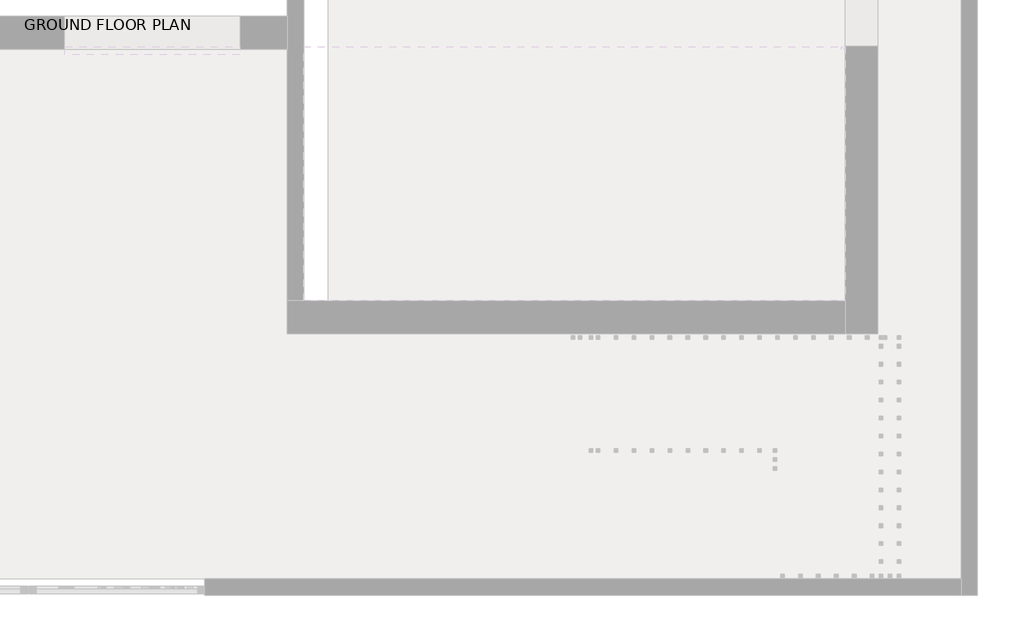
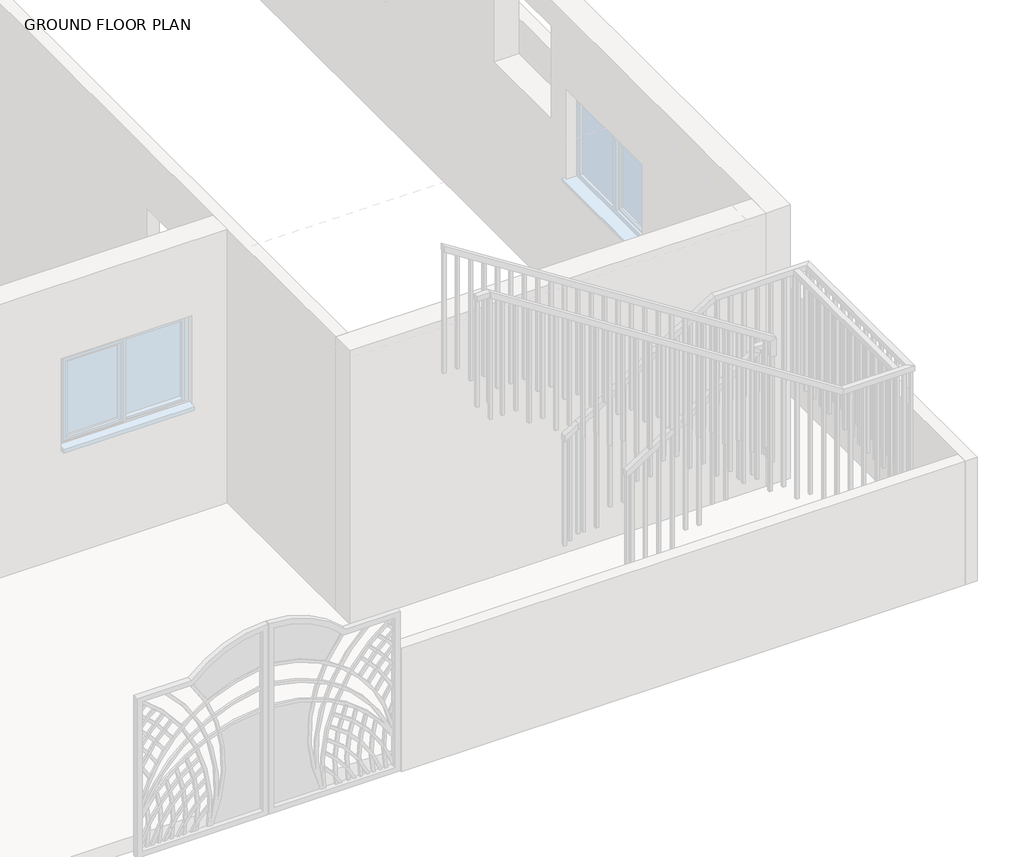
# One storey, part 8 of 23: 2 railings.
"""IFC4 building model written with IfcOpenShell, lengths in millimetres."""

from ifc_helpers import new_model, si_unit, frame, origin, place, context, project, spatial, polyline, outline, extrude, faceted_brep, element, save

model = new_model("IFC4")

# Units and contexts
model_context = context("Model", 3, world=origin())
ifc_project = project(units=[si_unit("LENGTHUNIT", "METRE", prefix="MILLI")], contexts=[model_context])

# Site, building, storey
site = spatial("IfcSite", under=ifc_project)
building = spatial("IfcBuilding", under=site)
storey = spatial("IfcBuildingStorey", under=building, Name="GROUND FLOOR PLAN", Elevation=487.68)

# Railings
placement = place(None, origin())
element("IfcRailing", 1, ObjectType="1100mm", at=placement, inside=storey, context=model_context, shape_type="SolidModel", body=[
    faceted_brep([(-8680.149573, -10220.0521308, 1912.8), (-8680.149573, -10220.0521308, 1853.4423995), (-8680.149573, -10270.0521308, 1853.4423995), (-8680.149573, -10270.0521308, 1912.8), (-7409.7306254, -10220.0521308, 2725.6), (-7395.1045513, -10220.0521308, 2675.6), (-7395.1045513, -10270.0521308, 2675.6), (-7409.7306254, -10270.0521308, 2725.6), (-6495.8132565, -10220.0521308, 2725.6), (-6495.8132565, -10220.0521308, 2675.6), (-6545.8132565, -10270.0521308, 2675.6), (-6545.8132565, -10270.0521308, 2725.6), (-6495.8132565, -11933.6860066, 2725.6), (-6495.8132565, -11933.6860066, 2675.6), (-6545.8132565, -11883.6860066, 2675.6), (-6545.8132565, -11883.6860066, 2725.6), (-7155.718398, -11933.6860066, 2725.6), (-7170.3479429, -11933.6860066, 2675.6), (-7170.3479429, -11883.6860066, 2675.6), (-7155.718398, -11883.6860066, 2725.6), (-10457.8773536, -11933.6860066, 4838.88), (-10457.8773536, -11883.6860066, 4838.88), (-10457.8773536, -11883.6860066, 4779.517542), (-10457.8773536, -11933.6860066, 4779.517542)], [[[0, 1, 2, 3]], [[1, 0, 4, 5]], [[2, 1, 5, 6]], [[3, 2, 6, 7]], [[0, 3, 7, 4]], [[5, 4, 8, 9]], [[6, 5, 9, 10]], [[7, 6, 10, 11]], [[4, 7, 11, 8]], [[9, 8, 12, 13]], [[10, 9, 13, 14]], [[11, 10, 14, 15]], [[8, 11, 15, 12]], [[13, 12, 16, 17]], [[14, 13, 17, 18]], [[15, 14, 18, 19]], [[12, 15, 19, 16]], [[20, 21, 22, 23]], [[17, 16, 20, 23]], [[18, 17, 23, 22]], [[19, 18, 22, 21]], [[16, 19, 21, 20]]]),
    extrude(outline(polyline([(4691.8007425, -10320.8132565), (4707.7999723, -10345.8132565), (3576.32, -10345.8132565), (3576.32, -10320.8132565), (4691.8007425, -10320.8132565)])), frame((0.0, -11921.1860066, 0.0), z_axis=(0.0, 1.0, 0.0), x_axis=(0.0, 0.0, 1.0)), (0.0, 0.0, 1.0), 25.0),
    extrude(outline(polyline([(4611.8045935, -10195.8132565), (4627.8038233, -10220.8132565), (3576.32, -10220.8132565), (3576.32, -10195.8132565), (4611.8045935, -10195.8132565)])), frame((0.0, -11921.1860066, 0.0), z_axis=(0.0, 1.0, 0.0), x_axis=(0.0, 0.0, 1.0)), (0.0, 0.0, 1.0), 25.0),
    extrude(outline(polyline([(4531.8084444, -10070.8132565), (4547.8076742, -10095.8132565), (3413.76, -10095.8132565), (3413.76, -10070.8132565), (4531.8084444, -10070.8132565)])), frame((0.0, -11921.1860066, 0.0), z_axis=(0.0, 1.0, 0.0), x_axis=(0.0, 0.0, 1.0)), (0.0, 0.0, 1.0), 25.0),
    extrude(outline(polyline([(4451.8122954, -9945.8132565), (4467.8115252, -9970.8132565), (3413.76, -9970.8132565), (3413.76, -9945.8132565), (4451.8122954, -9945.8132565)])), frame((0.0, -11921.1860066, 0.0), z_axis=(0.0, 1.0, 0.0), x_axis=(0.0, 0.0, 1.0)), (0.0, 0.0, 1.0), 25.0),
    extrude(outline(polyline([(4371.8161463, -9820.8132565), (4387.8153761, -9845.8132565), (3251.2, -9845.8132565), (3251.2, -9820.8132565), (4371.8161463, -9820.8132565)])), frame((0.0, -11921.1860066, 0.0), z_axis=(0.0, 1.0, 0.0), x_axis=(0.0, 0.0, 1.0)), (0.0, 0.0, 1.0), 25.0),
    extrude(outline(polyline([(4291.8423995, -9695.8132565), (4307.8371231, -9720.8132565), (3251.2, -9720.8132565), (3251.2, -9695.8132565), (4291.8423995, -9695.8132565)])), frame((0.0, -11921.1860066, 0.0), z_axis=(0.0, 1.0, 0.0), x_axis=(0.0, 0.0, 1.0)), (0.0, 0.0, 1.0), 25.0),
    extrude(outline(polyline([(4211.8238482, -9570.8132565), (4227.823078, -9595.8132565), (3088.64, -9595.8132565), (3088.64, -9570.8132565), (4211.8238482, -9570.8132565)])), frame((0.0, -11921.1860066, 0.0), z_axis=(0.0, 1.0, 0.0), x_axis=(0.0, 0.0, 1.0)), (0.0, 0.0, 1.0), 25.0),
    extrude(outline(polyline([(4131.8276992, -9445.8132565), (4147.826929, -9470.8132565), (3088.64, -9470.8132565), (3088.64, -9445.8132565), (4131.8276992, -9445.8132565)])), frame((0.0, -11921.1860066, 0.0), z_axis=(0.0, 1.0, 0.0), x_axis=(0.0, 0.0, 1.0)), (0.0, 0.0, 1.0), 25.0),
    extrude(outline(polyline([(4051.8315501, -9320.8132565), (4067.8307799, -9345.8132565), (2926.08, -9345.8132565), (2926.08, -9320.8132565), (4051.8315501, -9320.8132565)])), frame((0.0, -11921.1860066, 0.0), z_axis=(0.0, 1.0, 0.0), x_axis=(0.0, 0.0, 1.0)), (0.0, 0.0, 1.0), 25.0),
    extrude(outline(polyline([(3971.835401, -9195.8132565), (3987.8346309, -9220.8132565), (2926.08, -9220.8132565), (2926.08, -9195.8132565), (3971.835401, -9195.8132565)])), frame((0.0, -11921.1860066, 0.0), z_axis=(0.0, 1.0, 0.0), x_axis=(0.0, 0.0, 1.0)), (0.0, 0.0, 1.0), 25.0),
    extrude(outline(polyline([(3891.839252, -9070.8132565), (3907.8384818, -9095.8132565), (2763.52, -9095.8132565), (2763.52, -9070.8132565), (3891.839252, -9070.8132565)])), frame((0.0, -11921.1860066, 0.0), z_axis=(0.0, 1.0, 0.0), x_axis=(0.0, 0.0, 1.0)), (0.0, 0.0, 1.0), 25.0),
    extrude(outline(polyline([(3811.8431029, -8945.8132565), (3827.8423328, -8970.8132565), (2763.52, -8970.8132565), (2763.52, -8945.8132565), (3811.8431029, -8945.8132565)])), frame((0.0, -11921.1860066, 0.0), z_axis=(0.0, 1.0, 0.0), x_axis=(0.0, 0.0, 1.0)), (0.0, 0.0, 1.0), 25.0),
    extrude(outline(polyline([(3731.8469539, -8820.8132565), (3747.8461837, -8845.8132565), (2600.96, -8845.8132565), (2600.96, -8820.8132565), (3731.8469539, -8820.8132565)])), frame((0.0, -11921.1860066, 0.0), z_axis=(0.0, 1.0, 0.0), x_axis=(0.0, 0.0, 1.0)), (0.0, 0.0, 1.0), 25.0),
    extrude(outline(polyline([(3651.8508048, -8695.8132565), (3667.8500347, -8720.8132565), (2600.96, -8720.8132565), (2600.96, -8695.8132565), (3651.8508048, -8695.8132565)])), frame((0.0, -11921.1860066, 0.0), z_axis=(0.0, 1.0, 0.0), x_axis=(0.0, 0.0, 1.0)), (0.0, 0.0, 1.0), 25.0),
    extrude(outline(polyline([(3571.8546558, -8570.8132565), (3587.8538856, -8595.8132565), (2438.4, -8595.8132565), (2438.4, -8570.8132565), (3571.8546558, -8570.8132565)])), frame((0.0, -11921.1860066, 0.0), z_axis=(0.0, 1.0, 0.0), x_axis=(0.0, 0.0, 1.0)), (0.0, 0.0, 1.0), 25.0),
    extrude(outline(polyline([(3491.8585067, -8445.8132565), (3507.8577365, -8470.8132565), (2438.4, -8470.8132565), (2438.4, -8445.8132565), (3491.8585067, -8445.8132565)])), frame((0.0, -11921.1860066, 0.0), z_axis=(0.0, 1.0, 0.0), x_axis=(0.0, 0.0, 1.0)), (0.0, 0.0, 1.0), 25.0),
    extrude(outline(polyline([(3411.8623577, -8320.8132565), (3427.8615875, -8345.8132565), (2275.84, -8345.8132565), (2275.84, -8320.8132565), (3411.8623577, -8320.8132565)])), frame((0.0, -11921.1860066, 0.0), z_axis=(0.0, 1.0, 0.0), x_axis=(0.0, 0.0, 1.0)), (0.0, 0.0, 1.0), 25.0),
    extrude(outline(polyline([(3331.8662086, -8195.8132565), (3347.8654384, -8220.8132565), (2275.84, -8220.8132565), (2275.84, -8195.8132565), (3331.8662086, -8195.8132565)])), frame((0.0, -11921.1860066, 0.0), z_axis=(0.0, 1.0, 0.0), x_axis=(0.0, 0.0, 1.0)), (0.0, 0.0, 1.0), 25.0),
    extrude(outline(polyline([(3251.8700596, -8070.8132565), (3267.8692894, -8095.8132565), (2113.28, -8095.8132565), (2113.28, -8070.8132565), (3251.8700596, -8070.8132565)])), frame((0.0, -11921.1860066, 0.0), z_axis=(0.0, 1.0, 0.0), x_axis=(0.0, 0.0, 1.0)), (0.0, 0.0, 1.0), 25.0),
    extrude(outline(polyline([(3171.8739105, -7945.8132565), (3187.8731403, -7970.8132565), (2113.28, -7970.8132565), (2113.28, -7945.8132565), (3171.8739105, -7945.8132565)])), frame((0.0, -11921.1860066, 0.0), z_axis=(0.0, 1.0, 0.0), x_axis=(0.0, 0.0, 1.0)), (0.0, 0.0, 1.0), 25.0),
    extrude(outline(polyline([(3091.8777615, -7820.8132565), (3107.8769913, -7845.8132565), (1950.72, -7845.8132565), (1950.72, -7820.8132565), (3091.8777615, -7820.8132565)])), frame((0.0, -11921.1860066, 0.0), z_axis=(0.0, 1.0, 0.0), x_axis=(0.0, 0.0, 1.0)), (0.0, 0.0, 1.0), 25.0),
    extrude(outline(polyline([(3011.8816124, -7695.8132565), (3027.8808422, -7720.8132565), (1950.72, -7720.8132565), (1950.72, -7695.8132565), (3011.8816124, -7695.8132565)])), frame((0.0, -11921.1860066, 0.0), z_axis=(0.0, 1.0, 0.0), x_axis=(0.0, 0.0, 1.0)), (0.0, 0.0, 1.0), 25.0),
    extrude(outline(polyline([(2931.8854634, -7570.8132565), (2947.8846932, -7595.8132565), (1788.16, -7595.8132565), (1788.16, -7570.8132565), (2931.8854634, -7570.8132565)])), frame((0.0, -11921.1860066, 0.0), z_axis=(0.0, 1.0, 0.0), x_axis=(0.0, 0.0, 1.0)), (0.0, 0.0, 1.0), 25.0),
    extrude(outline(polyline([(2851.8893143, -7445.8132565), (2867.8885441, -7470.8132565), (1788.16, -7470.8132565), (1788.16, -7445.8132565), (2851.8893143, -7445.8132565)])), frame((0.0, -11921.1860066, 0.0), z_axis=(0.0, 1.0, 0.0), x_axis=(0.0, 0.0, 1.0)), (0.0, 0.0, 1.0), 25.0),
    extrude(outline(polyline([(2771.8931653, -7320.8132565), (2787.8923951, -7345.8132565), (1625.6, -7345.8132565), (1625.6, -7320.8132565), (2771.8931653, -7320.8132565)])), frame((0.0, -11921.1860066, 0.0), z_axis=(0.0, 1.0, 0.0), x_axis=(0.0, 0.0, 1.0)), (0.0, 0.0, 1.0), 25.0),
    extrude(outline(polyline([(2691.8970162, -7195.8132565), (2707.896246, -7220.8132565), (1625.6, -7220.8132565), (1625.6, -7195.8132565), (2691.8970162, -7195.8132565)])), frame((0.0, -11921.1860066, 0.0), z_axis=(0.0, 1.0, 0.0), x_axis=(0.0, 0.0, 1.0)), (0.0, 0.0, 1.0), 25.0),
    extrude(outline(polyline([(-7070.8132565, -11921.1860066), (-7095.8132565, -11921.1860066), (-7095.8132565, -11896.1860066), (-7070.8132565, -11896.1860066), (-7070.8132565, -11921.1860066)])), frame((0.0, 0.0, 1625.6), z_axis=(0.0, 0.0, 1.0), x_axis=(1.0, 0.0, 0.0)), (0.0, 0.0, 1.0), 1050.0),
    extrude(outline(polyline([(-6945.8132565, -11921.1860066), (-6970.8132565, -11921.1860066), (-6970.8132565, -11896.1860066), (-6945.8132565, -11896.1860066), (-6945.8132565, -11921.1860066)])), frame((0.0, 0.0, 1625.6), z_axis=(0.0, 0.0, 1.0), x_axis=(1.0, 0.0, 0.0)), (0.0, 0.0, 1.0), 1050.0),
    extrude(outline(polyline([(-6820.8132565, -11921.1860066), (-6845.8132565, -11921.1860066), (-6845.8132565, -11896.1860066), (-6820.8132565, -11896.1860066), (-6820.8132565, -11921.1860066)])), frame((0.0, 0.0, 1625.6), z_axis=(0.0, 0.0, 1.0), x_axis=(1.0, 0.0, 0.0)), (0.0, 0.0, 1.0), 1050.0),
    extrude(outline(polyline([(-6695.8132565, -11921.1860066), (-6720.8132565, -11921.1860066), (-6720.8132565, -11896.1860066), (-6695.8132565, -11896.1860066), (-6695.8132565, -11921.1860066)])), frame((0.0, 0.0, 1625.6), z_axis=(0.0, 0.0, 1.0), x_axis=(1.0, 0.0, 0.0)), (0.0, 0.0, 1.0), 1050.0),
    extrude(outline(polyline([(-6570.8132565, -11921.1860066), (-6595.8132565, -11921.1860066), (-6595.8132565, -11896.1860066), (-6570.8132565, -11896.1860066), (-6570.8132565, -11921.1860066)])), frame((0.0, 0.0, 1625.6), z_axis=(0.0, 0.0, 1.0), x_axis=(1.0, 0.0, 0.0)), (0.0, 0.0, 1.0), 1050.0),
    extrude(outline(polyline([(-6508.3132565, -11795.0521308), (-6508.3132565, -11820.0521308), (-6533.3132565, -11820.0521308), (-6533.3132565, -11795.0521308), (-6508.3132565, -11795.0521308)])), frame((0.0, 0.0, 1625.6), z_axis=(0.0, 0.0, 1.0), x_axis=(1.0, 0.0, 0.0)), (0.0, 0.0, 1.0), 1050.0),
    extrude(outline(polyline([(-6508.3132565, -11670.0521308), (-6508.3132565, -11695.0521308), (-6533.3132565, -11695.0521308), (-6533.3132565, -11670.0521308), (-6508.3132565, -11670.0521308)])), frame((0.0, 0.0, 1625.6), z_axis=(0.0, 0.0, 1.0), x_axis=(1.0, 0.0, 0.0)), (0.0, 0.0, 1.0), 1050.0),
    extrude(outline(polyline([(-6508.3132565, -11545.0521308), (-6508.3132565, -11570.0521308), (-6533.3132565, -11570.0521308), (-6533.3132565, -11545.0521308), (-6508.3132565, -11545.0521308)])), frame((0.0, 0.0, 1625.6), z_axis=(0.0, 0.0, 1.0), x_axis=(1.0, 0.0, 0.0)), (0.0, 0.0, 1.0), 1050.0),
    extrude(outline(polyline([(-6508.3132565, -11420.0521308), (-6508.3132565, -11445.0521308), (-6533.3132565, -11445.0521308), (-6533.3132565, -11420.0521308), (-6508.3132565, -11420.0521308)])), frame((0.0, 0.0, 1625.6), z_axis=(0.0, 0.0, 1.0), x_axis=(1.0, 0.0, 0.0)), (0.0, 0.0, 1.0), 1050.0),
    extrude(outline(polyline([(-6508.3132565, -11295.0521308), (-6508.3132565, -11320.0521308), (-6533.3132565, -11320.0521308), (-6533.3132565, -11295.0521308), (-6508.3132565, -11295.0521308)])), frame((0.0, 0.0, 1625.6), z_axis=(0.0, 0.0, 1.0), x_axis=(1.0, 0.0, 0.0)), (0.0, 0.0, 1.0), 1050.0),
    extrude(outline(polyline([(-6508.3132565, -11170.0521308), (-6508.3132565, -11195.0521308), (-6533.3132565, -11195.0521308), (-6533.3132565, -11170.0521308), (-6508.3132565, -11170.0521308)])), frame((0.0, 0.0, 1625.6), z_axis=(0.0, 0.0, 1.0), x_axis=(1.0, 0.0, 0.0)), (0.0, 0.0, 1.0), 1050.0),
    extrude(outline(polyline([(-6508.3132565, -11045.0521308), (-6508.3132565, -11070.0521308), (-6533.3132565, -11070.0521308), (-6533.3132565, -11045.0521308), (-6508.3132565, -11045.0521308)])), frame((0.0, 0.0, 1625.6), z_axis=(0.0, 0.0, 1.0), x_axis=(1.0, 0.0, 0.0)), (0.0, 0.0, 1.0), 1050.0),
    extrude(outline(polyline([(-6508.3132565, -10920.0521308), (-6508.3132565, -10945.0521308), (-6533.3132565, -10945.0521308), (-6533.3132565, -10920.0521308), (-6508.3132565, -10920.0521308)])), frame((0.0, 0.0, 1625.6), z_axis=(0.0, 0.0, 1.0), x_axis=(1.0, 0.0, 0.0)), (0.0, 0.0, 1.0), 1050.0),
    extrude(outline(polyline([(-6508.3132565, -10795.0521308), (-6508.3132565, -10820.0521308), (-6533.3132565, -10820.0521308), (-6533.3132565, -10795.0521308), (-6508.3132565, -10795.0521308)])), frame((0.0, 0.0, 1625.6), z_axis=(0.0, 0.0, 1.0), x_axis=(1.0, 0.0, 0.0)), (0.0, 0.0, 1.0), 1050.0),
    extrude(outline(polyline([(-6508.3132565, -10670.0521308), (-6508.3132565, -10695.0521308), (-6533.3132565, -10695.0521308), (-6533.3132565, -10670.0521308), (-6508.3132565, -10670.0521308)])), frame((0.0, 0.0, 1625.6), z_axis=(0.0, 0.0, 1.0), x_axis=(1.0, 0.0, 0.0)), (0.0, 0.0, 1.0), 1050.0),
    extrude(outline(polyline([(-6508.3132565, -10545.0521308), (-6508.3132565, -10570.0521308), (-6533.3132565, -10570.0521308), (-6533.3132565, -10545.0521308), (-6508.3132565, -10545.0521308)])), frame((0.0, 0.0, 1625.6), z_axis=(0.0, 0.0, 1.0), x_axis=(1.0, 0.0, 0.0)), (0.0, 0.0, 1.0), 1050.0),
    extrude(outline(polyline([(-6508.3132565, -10420.0521308), (-6508.3132565, -10445.0521308), (-6533.3132565, -10445.0521308), (-6533.3132565, -10420.0521308), (-6508.3132565, -10420.0521308)])), frame((0.0, 0.0, 1625.6), z_axis=(0.0, 0.0, 1.0), x_axis=(1.0, 0.0, 0.0)), (0.0, 0.0, 1.0), 1050.0),
    extrude(outline(polyline([(-6508.3132565, -10295.0521308), (-6508.3132565, -10320.0521308), (-6533.3132565, -10320.0521308), (-6533.3132565, -10295.0521308), (-6508.3132565, -10295.0521308)])), frame((0.0, 0.0, 1625.6), z_axis=(0.0, 0.0, 1.0), x_axis=(1.0, 0.0, 0.0)), (0.0, 0.0, 1.0), 1050.0),
    extrude(outline(polyline([(-6630.149573, -10232.5521308), (-6605.149573, -10232.5521308), (-6605.149573, -10257.5521308), (-6630.149573, -10257.5521308), (-6630.149573, -10232.5521308)])), frame((0.0, 0.0, 1625.6), z_axis=(0.0, 0.0, 1.0), x_axis=(1.0, 0.0, 0.0)), (0.0, 0.0, 1.0), 1050.0),
    extrude(outline(polyline([(-6755.149573, -10232.5521308), (-6730.149573, -10232.5521308), (-6730.149573, -10257.5521308), (-6755.149573, -10257.5521308), (-6755.149573, -10232.5521308)])), frame((0.0, 0.0, 1625.6), z_axis=(0.0, 0.0, 1.0), x_axis=(1.0, 0.0, 0.0)), (0.0, 0.0, 1.0), 1050.0),
    extrude(outline(polyline([(-6880.149573, -10232.5521308), (-6855.149573, -10232.5521308), (-6855.149573, -10257.5521308), (-6880.149573, -10257.5521308), (-6880.149573, -10232.5521308)])), frame((0.0, 0.0, 1625.6), z_axis=(0.0, 0.0, 1.0), x_axis=(1.0, 0.0, 0.0)), (0.0, 0.0, 1.0), 1050.0),
    extrude(outline(polyline([(-7005.149573, -10232.5521308), (-6980.149573, -10232.5521308), (-6980.149573, -10257.5521308), (-7005.149573, -10257.5521308), (-7005.149573, -10232.5521308)])), frame((0.0, 0.0, 1625.6), z_axis=(0.0, 0.0, 1.0), x_axis=(1.0, 0.0, 0.0)), (0.0, 0.0, 1.0), 1050.0),
    extrude(outline(polyline([(-7130.149573, -10232.5521308), (-7105.149573, -10232.5521308), (-7105.149573, -10257.5521308), (-7130.149573, -10257.5521308), (-7130.149573, -10232.5521308)])), frame((0.0, 0.0, 1625.6), z_axis=(0.0, 0.0, 1.0), x_axis=(1.0, 0.0, 0.0)), (0.0, 0.0, 1.0), 1050.0),
    extrude(outline(polyline([(-7255.149573, -10232.5521308), (-7230.149573, -10232.5521308), (-7230.149573, -10257.5521308), (-7255.149573, -10257.5521308), (-7255.149573, -10232.5521308)])), frame((0.0, 0.0, 1625.6), z_axis=(0.0, 0.0, 1.0), x_axis=(1.0, 0.0, 0.0)), (0.0, 0.0, 1.0), 1050.0),
    extrude(outline(polyline([(-7380.149573, -10232.5521308), (-7355.149573, -10232.5521308), (-7355.149573, -10257.5521308), (-7380.149573, -10257.5521308), (-7380.149573, -10232.5521308)])), frame((0.0, 0.0, 1625.6), z_axis=(0.0, 0.0, 1.0), x_axis=(1.0, 0.0, 0.0)), (0.0, 0.0, 1.0), 1050.0),
    extrude(outline(polyline([(1463.04, -7505.149573), (1463.04, -7480.149573), (2621.1891352, -7480.149573), (2605.1944115, -7505.149573), (1463.04, -7505.149573)])), frame((0.0, -10257.5521308, 0.0), z_axis=(0.0, 1.0, 0.0), x_axis=(0.0, 0.0, 1.0)), (0.0, 0.0, 1.0), 25.0),
    extrude(outline(polyline([(1463.04, -7630.149573), (1463.04, -7605.149573), (2541.2155169, -7605.149573), (2525.2207932, -7630.149573), (1463.04, -7630.149573)])), frame((0.0, -10257.5521308, 0.0), z_axis=(0.0, 1.0, 0.0), x_axis=(0.0, 0.0, 1.0)), (0.0, 0.0, 1.0), 25.0),
    extrude(outline(polyline([(1300.48, -7755.149573), (1300.48, -7730.149573), (2461.2418986, -7730.149573), (2445.2471749, -7755.149573), (1300.48, -7755.149573)])), frame((0.0, -10257.5521308, 0.0), z_axis=(0.0, 1.0, 0.0), x_axis=(0.0, 0.0, 1.0)), (0.0, 0.0, 1.0), 25.0),
    extrude(outline(polyline([(1300.48, -7880.149573), (1300.48, -7855.149573), (2381.2682803, -7855.149573), (2365.2735566, -7880.149573), (1300.48, -7880.149573)])), frame((0.0, -10257.5521308, 0.0), z_axis=(0.0, 1.0, 0.0), x_axis=(0.0, 0.0, 1.0)), (0.0, 0.0, 1.0), 25.0),
    extrude(outline(polyline([(1137.92, -8005.149573), (1137.92, -7980.149573), (2301.294662, -7980.149573), (2285.2999383, -8005.149573), (1137.92, -8005.149573)])), frame((0.0, -10257.5521308, 0.0), z_axis=(0.0, 1.0, 0.0), x_axis=(0.0, 0.0, 1.0)), (0.0, 0.0, 1.0), 25.0),
    extrude(outline(polyline([(1137.92, -8130.149573), (1137.92, -8105.149573), (2221.3210437, -8105.149573), (2205.32632, -8130.149573), (1137.92, -8130.149573)])), frame((0.0, -10257.5521308, 0.0), z_axis=(0.0, 1.0, 0.0), x_axis=(0.0, 0.0, 1.0)), (0.0, 0.0, 1.0), 25.0),
    extrude(outline(polyline([(975.36, -8255.149573), (975.36, -8230.149573), (2141.3474254, -8230.149573), (2125.3527017, -8255.149573), (975.36, -8255.149573)])), frame((0.0, -10257.5521308, 0.0), z_axis=(0.0, 1.0, 0.0), x_axis=(0.0, 0.0, 1.0)), (0.0, 0.0, 1.0), 25.0),
    extrude(outline(polyline([(975.36, -8380.149573), (975.36, -8355.149573), (2061.3738071, -8355.149573), (2045.3790834, -8380.149573), (975.36, -8380.149573)])), frame((0.0, -10257.5521308, 0.0), z_axis=(0.0, 1.0, 0.0), x_axis=(0.0, 0.0, 1.0)), (0.0, 0.0, 1.0), 25.0),
    extrude(outline(polyline([(812.8, -8505.149573), (812.8, -8480.149573), (1981.4001888, -8480.149573), (1965.4054651, -8505.149573), (812.8, -8505.149573)])), frame((0.0, -10257.5521308, 0.0), z_axis=(0.0, 1.0, 0.0), x_axis=(0.0, 0.0, 1.0)), (0.0, 0.0, 1.0), 25.0),
    extrude(outline(polyline([(812.8, -8630.149573), (812.8, -8605.149573), (1901.4265705, -8605.149573), (1885.4318468, -8630.149573), (812.8, -8630.149573)])), frame((0.0, -10257.5521308, 0.0), z_axis=(0.0, 1.0, 0.0), x_axis=(0.0, 0.0, 1.0)), (0.0, 0.0, 1.0), 25.0),
    extrude(outline(polyline([(-6508.3132565, -11896.1860066), (-6508.3132565, -11921.1860066), (-6533.3132565, -11921.1860066), (-6533.3132565, -11896.1860066), (-6508.3132565, -11896.1860066)])), frame((0.0, 0.0, 1625.6), z_axis=(0.0, 0.0, 1.0), x_axis=(1.0, 0.0, 0.0)), (0.0, 0.0, 1.0), 1050.0),
    extrude(outline(polyline([(-6533.3132565, -10232.5521308), (-6508.3132565, -10232.5521308), (-6508.3132565, -10257.5521308), (-6533.3132565, -10257.5521308), (-6533.3132565, -10232.5521308)])), frame((0.0, 0.0, 1625.6), z_axis=(0.0, 0.0, 1.0), x_axis=(1.0, 0.0, 0.0)), (0.0, 0.0, 1.0), 1050.0),
    extrude(outline(polyline([(4763.5183122, -10432.8773536), (4779.517542, -10457.8773536), (3576.32, -10457.8773536), (3576.32, -10432.8773536), (4763.5183122, -10432.8773536)])), frame((0.0, -11921.1860066, 0.0), z_axis=(0.0, 1.0, 0.0), x_axis=(0.0, 0.0, 1.0)), (0.0, 0.0, 1.0), 25.0),
    extrude(outline(polyline([(812.8, -8680.149573), (812.8, -8655.149573), (1869.4371231, -8655.149573), (1853.4423995, -8680.149573), (812.8, -8680.149573)])), frame((0.0, -10257.5521308, 0.0), z_axis=(0.0, 1.0, 0.0), x_axis=(0.0, 0.0, 1.0)), (0.0, 0.0, 1.0), 25.0),
])
element("IfcRailing", 2, ObjectType="1100mm", at=placement, inside=storey, context=model_context, shape_type="SolidModel", body=[
    faceted_brep([(-8680.149573, -11007.9255223, 1912.8), (-8680.149573, -11007.9255223, 1853.4423995), (-8680.149573, -11057.9255223, 1853.4423995), (-8680.149573, -11057.9255223, 1912.8), (-7484.3306254, -11007.9255223, 2677.8717446), (-7434.3306254, -11007.9255223, 2650.5035914), (-7434.3306254, -11057.9255223, 2650.5035914), (-7484.3306254, -11057.9255223, 2677.8717446), (-7484.3306254, -11007.9255223, 2725.6), (-7434.3306254, -11007.9255223, 2675.6), (-7434.3306254, -11057.9255223, 2675.6), (-7484.3306254, -11057.9255223, 2725.6), (-7359.3306254, -11007.9255223, 2725.6), (-7359.3306254, -11007.9255223, 2675.6), (-7409.3306254, -11057.9255223, 2675.6), (-7409.3306254, -11057.9255223, 2725.6), (-7359.3306254, -11132.9255223, 2725.6), (-7359.3306254, -11132.9255223, 2675.6), (-7409.3306254, -11132.9255223, 2675.6), (-7409.3306254, -11132.9255223, 2725.6), (-7359.3306254, -11134.9255223, 2725.6), (-7409.3306254, -11134.9255223, 2725.6), (-7409.3306254, -11184.9255223, 2675.6), (-7359.3306254, -11184.9255223, 2675.6)], [[[0, 1, 2, 3]], [[1, 0, 4, 5]], [[2, 1, 5, 6]], [[3, 2, 6, 7]], [[0, 3, 7, 4]], [[5, 4, 8, 9]], [[6, 5, 9, 10]], [[7, 6, 10, 11]], [[4, 7, 11, 8]], [[9, 8, 12, 13]], [[10, 9, 13, 14]], [[11, 10, 14, 15]], [[8, 11, 15, 12]], [[13, 12, 16, 17]], [[14, 13, 17, 18]], [[15, 14, 18, 19]], [[12, 15, 19, 16]], [[20, 21, 22, 23]], [[17, 16, 20, 23]], [[18, 17, 23, 22]], [[19, 18, 22, 21]], [[16, 19, 21, 20]]]),
    faceted_brep([(-7359.3306254, -11184.9255223, 2855.9055527), (-7409.3306254, -11184.9255223, 2828.5415543), (-7409.3306254, -11134.9255223, 2828.5415543), (-7359.3306254, -11134.9255223, 2855.9055527), (-10457.8773536, -11184.9255223, 4838.88), (-10457.8773536, -11134.9255223, 4838.88), (-10457.8773536, -11134.9255223, 4779.517542), (-10457.8773536, -11184.9255223, 4779.517542)], [[[0, 1, 2, 3]], [[4, 5, 6, 7]], [[1, 0, 4, 7]], [[2, 1, 7, 6]], [[3, 2, 6, 5]], [[0, 3, 5, 4]]]),
    faceted_brep([(-7359.3306254, -11134.9255223, 2725.6), (-7359.3306254, -11184.9255223, 2675.6), (-7409.3306254, -11184.9255223, 2675.6), (-7409.3306254, -11134.9255223, 2725.6), (-7359.3306254, -11134.9255223, 2855.9055527), (-7409.3306254, -11134.9255223, 2828.5415543), (-7409.3306254, -11184.9255223, 2828.5415543), (-7359.3306254, -11184.9255223, 2855.9055527)], [[[0, 1, 2, 3]], [[4, 5, 6, 7]], [[1, 0, 4, 7]], [[2, 1, 7, 6]], [[3, 2, 6, 5]], [[0, 3, 5, 4]]]),
    extrude(outline(polyline([(3576.32, -10434.3306254), (4764.4483614, -10434.3306254), (4780.4475912, -10459.3306254), (3576.32, -10459.3306254), (3576.32, -10434.3306254)])), frame((0.0, -11172.4255223, 0.0), z_axis=(0.0, 1.0, 0.0), x_axis=(0.0, 0.0, 1.0)), (0.0, 0.0, 1.0), 25.0),
    extrude(outline(polyline([(3576.32, -10309.3306254), (4684.4522123, -10309.3306254), (4700.4514422, -10334.3306254), (3576.32, -10334.3306254), (3576.32, -10309.3306254)])), frame((0.0, -11172.4255223, 0.0), z_axis=(0.0, 1.0, 0.0), x_axis=(0.0, 0.0, 1.0)), (0.0, 0.0, 1.0), 25.0),
    extrude(outline(polyline([(3413.76, -10184.3306254), (4604.4560633, -10184.3306254), (4620.4552931, -10209.3306254), (3413.76, -10209.3306254), (3413.76, -10184.3306254)])), frame((0.0, -11172.4255223, 0.0), z_axis=(0.0, 1.0, 0.0), x_axis=(0.0, 0.0, 1.0)), (0.0, 0.0, 1.0), 25.0),
    extrude(outline(polyline([(3413.76, -10059.3306254), (4524.4599142, -10059.3306254), (4540.459144, -10084.3306254), (3413.76, -10084.3306254), (3413.76, -10059.3306254)])), frame((0.0, -11172.4255223, 0.0), z_axis=(0.0, 1.0, 0.0), x_axis=(0.0, 0.0, 1.0)), (0.0, 0.0, 1.0), 25.0),
    extrude(outline(polyline([(3251.2, -9934.3306254), (4444.4637652, -9934.3306254), (4460.462995, -9959.3306254), (3251.2, -9959.3306254), (3251.2, -9934.3306254)])), frame((0.0, -11172.4255223, 0.0), z_axis=(0.0, 1.0, 0.0), x_axis=(0.0, 0.0, 1.0)), (0.0, 0.0, 1.0), 25.0),
    extrude(outline(polyline([(3251.2, -9809.3306254), (4364.4676161, -9809.3306254), (4380.4668459, -9834.3306254), (3251.2, -9834.3306254), (3251.2, -9809.3306254)])), frame((0.0, -11172.4255223, 0.0), z_axis=(0.0, 1.0, 0.0), x_axis=(0.0, 0.0, 1.0)), (0.0, 0.0, 1.0), 25.0),
    extrude(outline(polyline([(3251.2, -9684.3306254), (4284.4714671, -9684.3306254), (4300.4706969, -9709.3306254), (3251.2, -9709.3306254), (3251.2, -9684.3306254)])), frame((0.0, -11172.4255223, 0.0), z_axis=(0.0, 1.0, 0.0), x_axis=(0.0, 0.0, 1.0)), (0.0, 0.0, 1.0), 25.0),
    extrude(outline(polyline([(3088.64, -9559.3306254), (4204.475318, -9559.3306254), (4220.4745478, -9584.3306254), (3088.64, -9584.3306254), (3088.64, -9559.3306254)])), frame((0.0, -11172.4255223, 0.0), z_axis=(0.0, 1.0, 0.0), x_axis=(0.0, 0.0, 1.0)), (0.0, 0.0, 1.0), 25.0),
    extrude(outline(polyline([(3088.64, -9434.3306254), (4124.479169, -9434.3306254), (4140.4783988, -9459.3306254), (3088.64, -9459.3306254), (3088.64, -9434.3306254)])), frame((0.0, -11172.4255223, 0.0), z_axis=(0.0, 1.0, 0.0), x_axis=(0.0, 0.0, 1.0)), (0.0, 0.0, 1.0), 25.0),
    extrude(outline(polyline([(2926.08, -9309.3306254), (4044.4830199, -9309.3306254), (4060.4822497, -9334.3306254), (2926.08, -9334.3306254), (2926.08, -9309.3306254)])), frame((0.0, -11172.4255223, 0.0), z_axis=(0.0, 1.0, 0.0), x_axis=(0.0, 0.0, 1.0)), (0.0, 0.0, 1.0), 25.0),
    extrude(outline(polyline([(2926.08, -9184.3306254), (3964.4868709, -9184.3306254), (3980.4861007, -9209.3306254), (2926.08, -9209.3306254), (2926.08, -9184.3306254)])), frame((0.0, -11172.4255223, 0.0), z_axis=(0.0, 1.0, 0.0), x_axis=(0.0, 0.0, 1.0)), (0.0, 0.0, 1.0), 25.0),
    extrude(outline(polyline([(2763.52, -9059.3306254), (3884.4907218, -9059.3306254), (3900.4899516, -9084.3306254), (2763.52, -9084.3306254), (2763.52, -9059.3306254)])), frame((0.0, -11172.4255223, 0.0), z_axis=(0.0, 1.0, 0.0), x_axis=(0.0, 0.0, 1.0)), (0.0, 0.0, 1.0), 25.0),
    extrude(outline(polyline([(2763.52, -8934.3306254), (3804.4945728, -8934.3306254), (3820.4938026, -8959.3306254), (2763.52, -8959.3306254), (2763.52, -8934.3306254)])), frame((0.0, -11172.4255223, 0.0), z_axis=(0.0, 1.0, 0.0), x_axis=(0.0, 0.0, 1.0)), (0.0, 0.0, 1.0), 25.0),
    extrude(outline(polyline([(2600.96, -8809.3306254), (3724.4984237, -8809.3306254), (3740.4976535, -8834.3306254), (2600.96, -8834.3306254), (2600.96, -8809.3306254)])), frame((0.0, -11172.4255223, 0.0), z_axis=(0.0, 1.0, 0.0), x_axis=(0.0, 0.0, 1.0)), (0.0, 0.0, 1.0), 25.0),
    extrude(outline(polyline([(2600.96, -8684.3306254), (3644.5022747, -8684.3306254), (3660.5015045, -8709.3306254), (2600.96, -8709.3306254), (2600.96, -8684.3306254)])), frame((0.0, -11172.4255223, 0.0), z_axis=(0.0, 1.0, 0.0), x_axis=(0.0, 0.0, 1.0)), (0.0, 0.0, 1.0), 25.0),
    extrude(outline(polyline([(2438.4, -8559.3306254), (3564.5061256, -8559.3306254), (3580.5053554, -8584.3306254), (2438.4, -8584.3306254), (2438.4, -8559.3306254)])), frame((0.0, -11172.4255223, 0.0), z_axis=(0.0, 1.0, 0.0), x_axis=(0.0, 0.0, 1.0)), (0.0, 0.0, 1.0), 25.0),
    extrude(outline(polyline([(2438.4, -8434.3306254), (3484.5099766, -8434.3306254), (3500.5092064, -8459.3306254), (2438.4, -8459.3306254), (2438.4, -8434.3306254)])), frame((0.0, -11172.4255223, 0.0), z_axis=(0.0, 1.0, 0.0), x_axis=(0.0, 0.0, 1.0)), (0.0, 0.0, 1.0), 25.0),
    extrude(outline(polyline([(2275.84, -8309.3306254), (3404.5138275, -8309.3306254), (3420.5130573, -8334.3306254), (2275.84, -8334.3306254), (2275.84, -8309.3306254)])), frame((0.0, -11172.4255223, 0.0), z_axis=(0.0, 1.0, 0.0), x_axis=(0.0, 0.0, 1.0)), (0.0, 0.0, 1.0), 25.0),
    extrude(outline(polyline([(2275.84, -8184.3306254), (3324.5176785, -8184.3306254), (3340.5169083, -8209.3306254), (2275.84, -8209.3306254), (2275.84, -8184.3306254)])), frame((0.0, -11172.4255223, 0.0), z_axis=(0.0, 1.0, 0.0), x_axis=(0.0, 0.0, 1.0)), (0.0, 0.0, 1.0), 25.0),
    extrude(outline(polyline([(2113.28, -8059.3306254), (3244.5215294, -8059.3306254), (3260.5207592, -8084.3306254), (2113.28, -8084.3306254), (2113.28, -8059.3306254)])), frame((0.0, -11172.4255223, 0.0), z_axis=(0.0, 1.0, 0.0), x_axis=(0.0, 0.0, 1.0)), (0.0, 0.0, 1.0), 25.0),
    extrude(outline(polyline([(2113.28, -7934.3306254), (3164.5253804, -7934.3306254), (3180.5246102, -7959.3306254), (2113.28, -7959.3306254), (2113.28, -7934.3306254)])), frame((0.0, -11172.4255223, 0.0), z_axis=(0.0, 1.0, 0.0), x_axis=(0.0, 0.0, 1.0)), (0.0, 0.0, 1.0), 25.0),
    extrude(outline(polyline([(1950.72, -7809.3306254), (3084.5292313, -7809.3306254), (3100.5284611, -7834.3306254), (1950.72, -7834.3306254), (1950.72, -7809.3306254)])), frame((0.0, -11172.4255223, 0.0), z_axis=(0.0, 1.0, 0.0), x_axis=(0.0, 0.0, 1.0)), (0.0, 0.0, 1.0), 25.0),
    extrude(outline(polyline([(1950.72, -7684.3306254), (3004.5330823, -7684.3306254), (3020.5323121, -7709.3306254), (1950.72, -7709.3306254), (1950.72, -7684.3306254)])), frame((0.0, -11172.4255223, 0.0), z_axis=(0.0, 1.0, 0.0), x_axis=(0.0, 0.0, 1.0)), (0.0, 0.0, 1.0), 25.0),
    extrude(outline(polyline([(1788.16, -7559.3306254), (2924.5369332, -7559.3306254), (2940.536163, -7584.3306254), (1788.16, -7584.3306254), (1788.16, -7559.3306254)])), frame((0.0, -11172.4255223, 0.0), z_axis=(0.0, 1.0, 0.0), x_axis=(0.0, 0.0, 1.0)), (0.0, 0.0, 1.0), 25.0),
    extrude(outline(polyline([(1788.16, -7434.3306254), (2844.5407841, -7434.3306254), (2860.540014, -7459.3306254), (1788.16, -7459.3306254), (1788.16, -7434.3306254)])), frame((0.0, -11172.4255223, 0.0), z_axis=(0.0, 1.0, 0.0), x_axis=(0.0, 0.0, 1.0)), (0.0, 0.0, 1.0), 25.0),
    extrude(outline(polyline([(-7396.8306254, -11082.9255223), (-7371.8306254, -11082.9255223), (-7371.8306254, -11107.9255223), (-7396.8306254, -11107.9255223), (-7396.8306254, -11082.9255223)])), frame((0.0, 0.0, 1625.6), z_axis=(0.0, 0.0, 1.0), x_axis=(1.0, 0.0, 0.0)), (0.0, 0.0, 1.0), 1050.0),
    extrude(outline(polyline([(2605.1944115, -7505.149573), (1463.04, -7505.149573), (1463.04, -7480.149573), (2621.1891352, -7480.149573), (2605.1944115, -7505.149573)])), frame((0.0, -11045.4255223, 0.0), z_axis=(0.0, 1.0, 0.0), x_axis=(0.0, 0.0, 1.0)), (0.0, 0.0, 1.0), 25.0),
    extrude(outline(polyline([(2525.2207932, -7630.149573), (1463.04, -7630.149573), (1463.04, -7605.149573), (2541.2155169, -7605.149573), (2525.2207932, -7630.149573)])), frame((0.0, -11045.4255223, 0.0), z_axis=(0.0, 1.0, 0.0), x_axis=(0.0, 0.0, 1.0)), (0.0, 0.0, 1.0), 25.0),
    extrude(outline(polyline([(2445.2471749, -7755.149573), (1300.48, -7755.149573), (1300.48, -7730.149573), (2461.2418986, -7730.149573), (2445.2471749, -7755.149573)])), frame((0.0, -11045.4255223, 0.0), z_axis=(0.0, 1.0, 0.0), x_axis=(0.0, 0.0, 1.0)), (0.0, 0.0, 1.0), 25.0),
    extrude(outline(polyline([(2365.2735566, -7880.149573), (1300.48, -7880.149573), (1300.48, -7855.149573), (2381.2682803, -7855.149573), (2365.2735566, -7880.149573)])), frame((0.0, -11045.4255223, 0.0), z_axis=(0.0, 1.0, 0.0), x_axis=(0.0, 0.0, 1.0)), (0.0, 0.0, 1.0), 25.0),
    extrude(outline(polyline([(2285.2999383, -8005.149573), (1137.92, -8005.149573), (1137.92, -7980.149573), (2301.294662, -7980.149573), (2285.2999383, -8005.149573)])), frame((0.0, -11045.4255223, 0.0), z_axis=(0.0, 1.0, 0.0), x_axis=(0.0, 0.0, 1.0)), (0.0, 0.0, 1.0), 25.0),
    extrude(outline(polyline([(2205.32632, -8130.149573), (1137.92, -8130.149573), (1137.92, -8105.149573), (2221.3210437, -8105.149573), (2205.32632, -8130.149573)])), frame((0.0, -11045.4255223, 0.0), z_axis=(0.0, 1.0, 0.0), x_axis=(0.0, 0.0, 1.0)), (0.0, 0.0, 1.0), 25.0),
    extrude(outline(polyline([(2125.3527017, -8255.149573), (975.36, -8255.149573), (975.36, -8230.149573), (2141.3474254, -8230.149573), (2125.3527017, -8255.149573)])), frame((0.0, -11045.4255223, 0.0), z_axis=(0.0, 1.0, 0.0), x_axis=(0.0, 0.0, 1.0)), (0.0, 0.0, 1.0), 25.0),
    extrude(outline(polyline([(2045.3790834, -8380.149573), (975.36, -8380.149573), (975.36, -8355.149573), (2061.3738071, -8355.149573), (2045.3790834, -8380.149573)])), frame((0.0, -11045.4255223, 0.0), z_axis=(0.0, 1.0, 0.0), x_axis=(0.0, 0.0, 1.0)), (0.0, 0.0, 1.0), 25.0),
    extrude(outline(polyline([(1965.4054651, -8505.149573), (812.8, -8505.149573), (812.8, -8480.149573), (1981.4001888, -8480.149573), (1965.4054651, -8505.149573)])), frame((0.0, -11045.4255223, 0.0), z_axis=(0.0, 1.0, 0.0), x_axis=(0.0, 0.0, 1.0)), (0.0, 0.0, 1.0), 25.0),
    extrude(outline(polyline([(1885.4318468, -8630.149573), (812.8, -8630.149573), (812.8, -8605.149573), (1901.4265705, -8605.149573), (1885.4318468, -8630.149573)])), frame((0.0, -11045.4255223, 0.0), z_axis=(0.0, 1.0, 0.0), x_axis=(0.0, 0.0, 1.0)), (0.0, 0.0, 1.0), 25.0),
    extrude(outline(polyline([(-7396.8306254, -11147.4255223), (-7371.8306254, -11147.4255223), (-7371.8306254, -11172.4255223), (-7396.8306254, -11172.4255223), (-7396.8306254, -11147.4255223)])), frame((0.0, 0.0, 1625.6), z_axis=(0.0, 0.0, 1.0), x_axis=(1.0, 0.0, 0.0)), (0.0, 0.0, 1.0), 1050.0),
    extrude(outline(polyline([(-7396.8306254, -11045.4255223), (-7396.8306254, -11020.4255223), (-7371.8306254, -11020.4255223), (-7371.8306254, -11045.4255223), (-7396.8306254, -11045.4255223)])), frame((0.0, 0.0, 1625.6), z_axis=(0.0, 0.0, 1.0), x_axis=(1.0, 0.0, 0.0)), (0.0, 0.0, 1.0), 1050.0),
    extrude(outline(polyline([(3576.32, -10432.8773536), (4763.5183122, -10432.8773536), (4779.517542, -10457.8773536), (3576.32, -10457.8773536), (3576.32, -10432.8773536)])), frame((0.0, -11172.4255223, 0.0), z_axis=(0.0, 1.0, 0.0), x_axis=(0.0, 0.0, 1.0)), (0.0, 0.0, 1.0), 25.0),
    extrude(outline(polyline([(1853.4423995, -8680.149573), (812.8, -8680.149573), (812.8, -8655.149573), (1869.4371231, -8655.149573), (1853.4423995, -8680.149573)])), frame((0.0, -11045.4255223, 0.0), z_axis=(0.0, 1.0, 0.0), x_axis=(0.0, 0.0, 1.0)), (0.0, 0.0, 1.0), 25.0),
])

save(model, "model.ifc")

# Revit data of these elements
# Type "1100mm"
#   built-in parameter 1008612 = 0.019685 (stored number, unit not read)
#   built-in parameter 1008611 = 0.019685 (stored number, unit not read)
#   built-in parameter 1008609 = 0.902231 (stored number, unit not read)
#   built-in parameter 1008604 = 0.19685 (stored number, unit not read)
#   built-in parameter 1008603 = 0.164042 (stored number, unit not read)
#   Railing Height = 3.608924 ft
#   built-in parameter 1008630 = 2
#   built-in parameter 1008610 = 2
#   built-in parameter 1008608 = 1
#   built-in parameter 1008618 = Baluster_Square : 25mm
# Elements 1, 2 (IfcRailing, "1100mm")
#   Phase Created = New Construction
